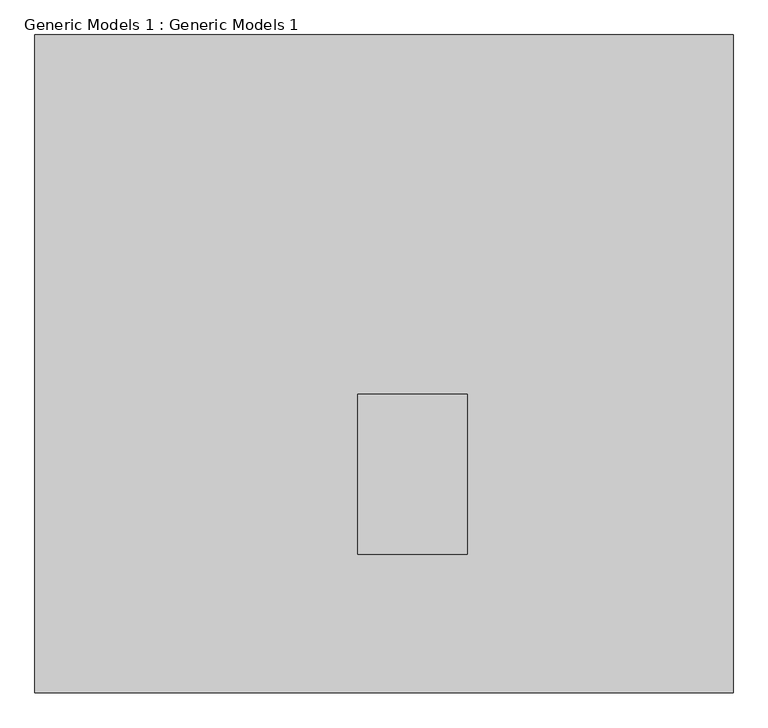
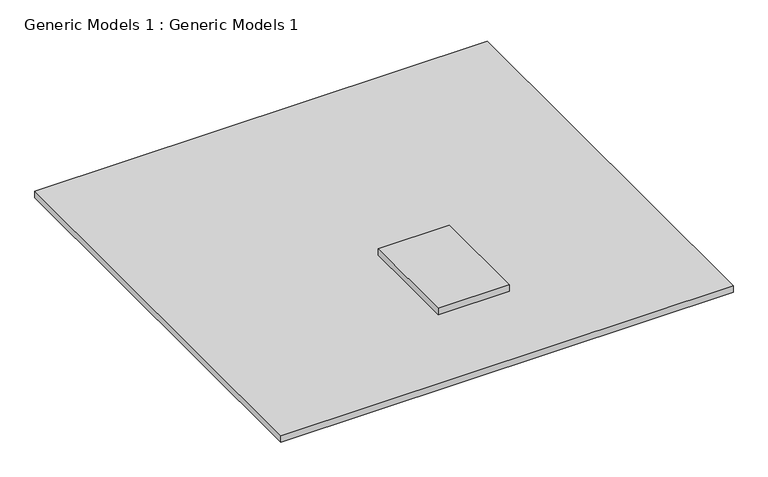
"""IFC4 building model written with IfcOpenShell, lengths in millimetres: proxy geometry, Generic Models 1 : Generic Models 1."""

from ifc_helpers import new_model, si_unit, frame, origin, origin_with_axes, place, context, project, spatial, polyline, outline, extrude, source, transform, mapped, element, save


def generic_models_1_generic_models_1_0bf7fa05(model_context):
    return source(origin(), model_context, "Body", "SweptSolid", [
        extrude(outline(polyline([(-1500.5760448, 1148.8495946), (-1500.5760448, -17805.3512614), (-21615.2648891, -17805.3512614), (-21615.2648891, 1148.8495946), (-1500.5760448, 1148.8495946)])), frame((0.0, 0.0, -304.8), z_axis=(0.0, 0.0, 1.0), x_axis=(1.0, 0.0, 0.0)), (0.0, 0.0, 1.0), 304.8),
        extrude(outline(polyline([(-9154.4628107, -9206.1642965), (-9154.4628107, -13816.2642965), (-12316.7628107, -13816.2642965), (-12316.7628107, -9206.1642965), (-9154.4628107, -9206.1642965)])), origin_with_axes(), (0.0, 0.0, 1.0), 304.8),
    ])


if __name__ == "__main__":
    model = new_model("IFC4")
    model_context = context("Model", 3, world=origin())
    ifc_project = project(units=[si_unit("LENGTHUNIT", "METRE", prefix="MILLI")], contexts=[model_context])
    site = spatial("IfcSite", under=ifc_project)
    building = spatial("IfcBuilding", under=site)
    placement = place(None, origin())
    generic_models_1_generic_models_1_shape = generic_models_1_generic_models_1_0bf7fa05(model_context)
    element("IfcBuildingElementProxy", 1, Name="Generic Models 1 : Generic Models 1", ObjectType="Generic Models 1 : Generic Models 1", at=placement, inside=building, context=model_context, shape_type="MappedRepresentation", body=[
        mapped(generic_models_1_generic_models_1_shape, transform((0.0, 0.0, 0.0), x_axis=(1.0, 0.0, 0.0), y_axis=(0.0, 1.0, 0.0), z_axis=(0.0, 0.0, 1.0))),
    ])
    save(model, "model.ifc")
